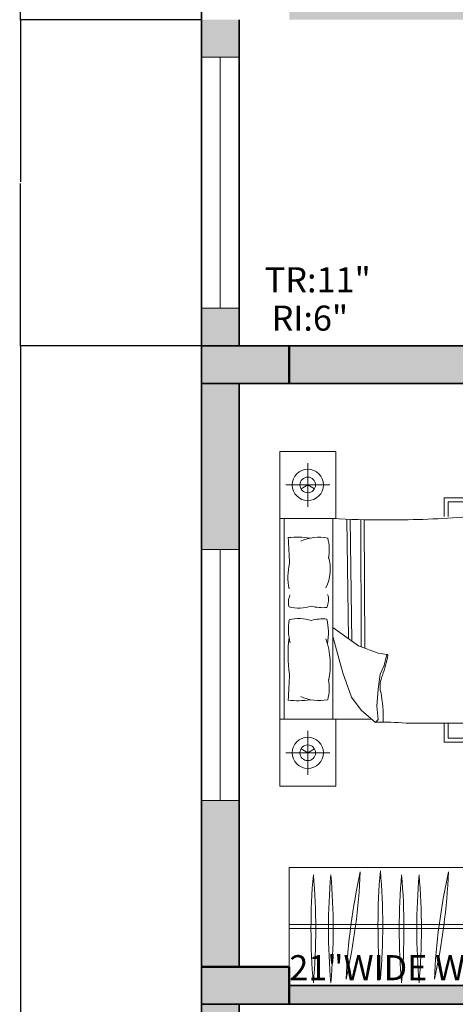
# Model space of a CAD drawing. Units: inches. Extents: x -28 to 485, y -861 to 54.
# Tile 2 of 14: x -28 to 76, y -600 to -365. Entities that reach past the tile are written whole.
import ezdxf

# ---------------------------------------------------------------- set-up
doc = ezdxf.new("R2010")
doc.units = ezdxf.units.IN
doc.header["$MEASUREMENT"] = 0
for name, color, linetype, lineweight in [('A-ANNO-DIMS', 2, 'Continuous', 18), ('A-ANNO-TEXT', 7, 'Continuous', 18), ('A-COLS', 7, 'Continuous', 50), ('A-COLS-PATT', 8, 'Continuous', 13), ('A-FLOR-CASE', 8, 'Continuous', 18), ('A-FURN', 8, 'Continuous', 13), ('A-GLAZ', 4, 'Continuous', 18), ('A-WALL', 7, 'Continuous', 35), ('A-WALL-PATT', 34, 'Continuous', 13)]:
    doc.layers.add(name, color=color, linetype=linetype, lineweight=lineweight)
doc.styles.get("Standard").update_dxf_attribs({"font": 'arial.ttf'})
doc.dimstyles.get("Standard").update_dxf_attribs({"dimtxt": 0.18, "dimasz": 0.18, "dimexe": 0.18, "dimexo": 0.0625, "dimgap": 0.09, "dimtad": 0, "dimtih": 1, "dimtoh": 1, "dimdec": 0, "dimzin": 0, "dimdsep": 46, "dimlunit": 3, "dimtxsty": 'Standard', "dimcen": 0.09, "dimadec": 0, "dimazin": 0, "dimtfac": 1, "dimtdec": 0, "dimtofl": 0, "dimtmove": 0, "dimatfit": 3, "dimfxl": 1, "dimtolj": 1, "dimtzin": 0, "dimarcsym": 0})

# ---------------------------------------------------------------- blocks, each defined once
blk = doc.blocks.new('BED-DOUBLE-WITH-NIGHTSTANDS')
for p, q in [((0, 0), (0, 80.08)), ((6.67, 66.84), (6.67, 77.31)), ((11.91, 72.08), (1.44, 72.08)), ((39.26, 64.51), (39.26, 68.96)), ((39.26, 68.96), (68.11, 68.96)), ((68.11, 68.96), (68.11, 10.57)), ((40.19, 68.03), (40.19, 64.5)), ((67.18, 68.03), (40.19, 68.03)), ((67.18, 11.5), (67.18, 68.03)), ((1.03, 64.07), (1.03, 16.02)), ((12.66, 16.02), (12.66, 64.07)), ((15.98, 63.85), (16.38, 35.34)), ((16.8, 63.82), (17.22, 34.74)), ((19.33, 63.78), (19.45, 33.37)), ((20.15, 63.78), (20.27, 33.06)), ((44.25, 64.43), (44.25, 15.09)), ((45.25, 64.51), (45.25, 15.09)), ((59.06, 60.14), (58.15, 60.31)), ((53.12, 56.3), (53.12, 23.78)), ((59.06, 54.54), (58.15, 54.36)), ((12.66, 38.02), (18.76, 33.63)), ((15.04, 27.14), (12.66, 35.87)), ((18.76, 33.63), (23.47, 31.84)), ((23.47, 31.84), (25.57, 31.52)), ((25.57, 31.52), (24.92, 28.93)), ((24.92, 28.93), (23.95, 26.82)), ((17.14, 21.3), (15.04, 27.14)), ((23.95, 26.82), (23.47, 23.25)), ((59.06, 24.99), (58.15, 25.16)), ((19.41, 18.22), (17.14, 21.3)), ((23.47, 23.25), (23.14, 19.19)), ((23.14, 19.19), (23.47, 15.95)), ((59.06, 19.39), (58.15, 19.21)), ((22.82, 15.3), (19.41, 18.22)), ((0, 16.02), (21.98, 16.02)), ((23.47, 15.95), (22.82, 15.3)), ((39.26, 10.57), (39.26, 15.1)), ((40.19, 15.1), (40.19, 11.5)), ((6.67, 13.24), (6.67, 2.78)), ((68.11, 10.57), (39.26, 10.57)), ((40.19, 11.5), (67.18, 11.5)), ((11.91, 8.01), (1.44, 8.01))]:
    blk.add_line(p, q)
for points in [[(0, 64.07), (13.35, 64.07), (13.35, 80.08), (0, 80.08)], [(6.67, 72.08), (5.06, 71.14)], [(6.67, 72.08), (8.29, 71.14)], [(13.35, 16.02), (13.35, 0), (0, 0)], [(6.67, 8.01), (5.06, 8.94)], [(6.67, 8.01), (8.29, 8.94)]]:
    blk.add_lwpolyline(points)
for points in [[(43.62, 64.41, 0.056112), (48.03, 64.99, 0.095341), (52.27, 66.12)], [(2, 59.47, -0.074897), (7.23, 59.37, 0.472817)], [(7.52, 43.09, -0.14099), (2.18, 42.93, -0.235245)], [(7.52, 39.67, 0.14099), (2.18, 39.83, 0.235245)], [(2, 20.62, 0.074897), (7.23, 20.71, -0.472817)], [(30.15, 15.13, 0.001242), (45.35, 15.09, -0.127202), (52.92, 13.49)]]:
    blk.add_lwpolyline(points, format="xyb")
for centre, radius in [((6.67, 72.08), 3.74), ((6.67, 72.08), 1.87), ((64.11, 56.84), 0.204), ((61.96, 55.51), 0.204), ((61.96, 24.02), 0.204), ((64.11, 22.68), 0.204), ((6.67, 8.01), 3.74), ((6.67, 8.01), 1.87)]:
    blk.add_circle(centre, radius)
for centre, radius, start, end in [((52.68, 65.51), 0.73, 336.5219, 123.8264), ((69.62, 57.92), 10.46, 111.4092, 145.6135), ((68.59, 75.81), 10.46, 228.1144, 262.255), ((69.99, 70.57), 5.1, 209.8884, 236.5383), ((70.94, 72.4), 6.35, 223.5186, 233.6964), ((22.44, 207.63), 143.9, 266.1, 270.9282), ((27.68, 251.44), 187.71, 269.1145, 274.8735), ((131.01, 58.75), 77.93, 175.2402, 181.8035), ((60.79, 62.99), 0.867, 76.272, 177.0484), ((59.47, 64.76), 1.79, 284.7031, 328.6173), ((61.96, 62.49), 1.65, 125.7657, 194.5347), ((53.85, 65.41), 7.32, 332.8176, 347.4827), ((61.24, 62.69), 1.16, 20.9613, 102.2885), ((61.86, 63.85), 0.873, 181.7131, 301.5367), ((59, 62.09), 2.64, 2.0648, 41.1598), ((60.59, 63.07), 0.856, 316.2238, 62.3173), ((68.81, 67.71), 4.25, 221.0454, 247.4453), ((66.52, 79.36), 14.47, 266.3481, 272.5919), ((58.76, 65.61), 6.06, 203.6453, 236.3329), ((55.85, 62.08), 1.35, 88.9462, 185.5144), ((56.85, 62.5), 2.41, 193.079, 274.7067), ((56.04, 61.53), 1.91, 7.1143, 95.0551), ((55.32, 60.77), 1.86, 338.5779, 68.4181), ((55.62, 61.86), 2.33, 305.9599, 357.6409), ((56.48, 64.35), 3.78, 288.2955, 328.7386), ((59.12, 61.97), 1.2, 19.1312, 189.736), ((58.76, 62.26), 1.5, 285.6955, 4.031), ((60.76, 60.64), 1.6, 128.4175, 173.8338), ((60.43, 62.21), 0.737, 126.7319, 206.0245), ((61.09, 62.57), 0.0682, 20.2667, 316.2271), ((61.51, 62.18), 0.13, 168.5166, 2.0648), ((61.45, 62.19), 0.0631, 52.0591, 168.5166), ((-760.15, 15.33), 763.42, 2.85022, 3.31479), ((9.33, 49.26), 10.32, 78.2417, 114.8684), ((1.06, 56.61), 10.73, 348.9631, 14.8961), ((54, 59.28), 0.964, 127.675, 162.5814), ((54, 59.28), 0.964, 196.6343, 225.5483), ((53.71, 63.39), 3.32, 259.249, 301.1782), ((54.57, 60.82), 2.55, 240.8249, 340.7178), ((53.81, 59.69), 1.2, 246.1646, 318.4347), ((55.15, 57.49), 3.09, 85.2696, 124.215), ((55.03, 61.2), 2.3, 240.0851, 262.564), ((55.94, 57.8), 1.64, 74.8529, 138.4347), ((57.33, 61.13), 1.99, 196.8663, 330.0915), ((56.5, 59.87), 0.497, 254.8529, 12.6959), ((55.15, 57.49), 3.09, 53.6555, 57.2989), ((56.78, 64.39), 4.3, 273.4924, 303.7117), ((60.19, 59.12), 0.158, 125.0752, 284.7644), ((60.43, 59.18), 0.34, 127.3642, 168.4363), ((60.17, 59.45), 0.49, 277.4968, 341.2737), ((60.56, 59.22), 0.195, 88.1325, 178.8919), ((60.95, 59.02), 0.422, 136.3462, 189.6513), ((60.71, 58.98), 0.176, 189.6513, 312.3208), ((60.75, 59.46), 0.204, 183.2768, 356.7232), ((61.39, 59.1), 0.668, 164.2829, 186.9148), ((60.6, 59.09), 0.334, 312.3208, 40.2111), ((61.31, 59.47), 0.474, 201.6382, 274.947), ((60.68, 58.82), 0.619, 42.3896, 66.5724), ((66.93, 63.72), 7.6, 217.9541, 226.8459), ((61.13, 59.18), 0.337, 10.9597, 52.2379), ((61.33, 59.15), 0.156, 274.947, 37.5263), ((57.16, 57.12), 0.251, 169.5864, 349.5616), ((57.25, 57.11), 0.154, 349.5616, 167.2949), ((61.28, 51.56), 6.63, 110.1059, 116.9968), ((59.06, 57.02), 0.42, 129.5056, 182.6421), ((57.85, 58), 1.27, 308.4388, 328.836), ((57.63, 59.02), 2.26, 296.5064, 305.3102), ((57.61, 57.86), 1.29, 336.3901, 344.4871), ((59.01, 57.53), 0.163, 83.9457, 185.6216), ((58.36, 57.69), 0.671, 328.836, 0.8141), ((58.71, 57.49), 0.384, 306.5232, 32.4668), ((59.16, 57.79), 0.163, 112.5583, 214.2343), ((59.06, 58.08), 0.384, 265.7131, 351.6568), ((58.72, 58.29), 0.671, 297.3659, 329.344), ((58.21, 58.87), 1.29, 313.6929, 321.7899), ((59.64, 57.99), 0.42, 115.5379, 168.6744), ((58.21, 58.6), 1.27, 329.344, 349.7412), ((61.28, 51.56), 6.63, 86.1723, 106.4158), ((57.2, 58.31), 2.26, 352.8698, 1.6736), ((61.66, 57.07), 0.93, 253.6301, 325.4631), ((61.86, 58.27), 0.163, 112.5583, 214.2343), ((61.75, 58.56), 0.384, 265.7131, 351.6568), ((61.42, 58.77), 0.671, 297.3659, 329.344), ((61.45, 54.86), 3.33, 60.7959, 85.244), ((54.37, 50.07), 10.94, 37.8256, 47.7588), ((60.91, 59.35), 1.29, 313.6929, 321.7899), ((61.87, 56.57), 0.565, 273.8774, 357.1501), ((62.33, 58.47), 0.42, 115.5379, 168.6744), ((60.9, 59.07), 1.27, 329.344, 349.7412), ((62.09, 56.97), 0.547, 262.0748, 308.2393), ((59.89, 58.78), 2.26, 352.8698, 1.6736), ((62.87, 56.86), 0.547, 215.1128, 261.2773), ((63.31, 56.83), 0.93, 197.889, 269.722), ((65.87, 54.52), 3.99, 130.182, 149.456), ((63.07, 58.33), 0.228, 33.0979, 123.1364), ((58.05, 55.12), 5.96, 31.1156, 34.8118), ((62.74, 57.94), 0.617, 2.3172, 70.5201), ((63.67, 56.79), 0.658, 139.3812, 199.9959), ((62.44, 57.27), 0.93, 310.9365, 22.7695), ((62.87, 57.22), 0.675, 285.6484, 332.2957), ((63.25, 57.78), 0.178, 135.7354, 318.1297), ((62.95, 58.07), 0.236, 315.7354, 31.1156), ((62.75, 57.57), 0.547, 319.3812, 5.5456), ((63.38, 57.79), 0.178, 68.2452, 250.6395), ((62.97, 58), 0.531, 352.6008, 57.1845), ((64.87, 54.44), 3.55, 111.7087, 116.2181), ((61.45, 54.86), 3.33, 47.5083, 55.9967), ((63.48, 58.12), 0.531, 252.8042, 349.6943), ((62.97, 57.17), 0.565, 331.1838, 51.6792), ((63.55, 56.5), 0.158, 125.0752, 284.7644), ((63.53, 58.17), 0.236, 248.2452, 323.6254), ((63.8, 56.56), 0.34, 93.635, 168.4363), ((63.33, 58.31), 0.617, 291.7087, 3.0299), ((63.75, 57.1), 0.2, 138.2946, 276.2474), ((63.53, 56.83), 0.49, 277.4968, 341.2737), ((63.83, 57.07), 0.278, 358.5719, 143.8954), ((58.93, 61.56), 5.96, 323.6254, 327.3216), ((63.92, 56.61), 0.195, 88.1325, 178.8919), ((63.99, 57.29), 0.281, 208.8493, 269.9355), ((63.75, 57.22), 0.321, 274.2123, 318.1587), ((64.31, 56.4), 0.422, 136.3462, 189.6513), ((63.81, 58.16), 0.228, 325.6077, 55.6462), ((64.75, 56.48), 0.668, 164.2829, 186.9148), ((64.73, 56.9), 0.643, 121.9501, 165.2442), ((63.96, 56.47), 0.334, 312.3208, 40.2111), ((64.67, 56.85), 0.474, 201.6382, 274.947), ((64.28, 57.14), 0.135, 262.868, 7.094), ((64.04, 56.2), 0.619, 42.3896, 66.5724), ((64.27, 57.26), 0.403, 278.5614, 22.5914), ((64.49, 56.56), 0.337, 10.9597, 118.7804), ((64.49, 57.27), 0.202, 44.3732, 121.9501), ((64.7, 56.53), 0.156, 274.947, 37.5263), ((1.85, 51.98), 10.19, 333.8761, 16.1746), ((54, 55.39), 0.964, 134.4517, 156.7144), ((54, 55.39), 0.964, 203.2856, 232.325), ((53.71, 51.28), 3.32, 58.8218, 100.2867), ((54.57, 53.85), 2.55, 19.2822, 119.1751), ((53.81, 54.99), 1.2, 41.5653, 113.8354), ((55.15, 57.18), 3.09, 235.785, 274.7304), ((55.03, 53.47), 2.3, 97.436, 119.9149), ((56.85, 52.18), 2.41, 85.2933, 166.921), ((55.94, 56.87), 1.64, 221.5653, 285.1471), ((57.33, 53.55), 1.99, 29.9085, 163.1337), ((55.32, 53.9), 1.86, 291.5819, 21.4221), ((56.5, 54.81), 0.497, 347.3041, 105.1471), ((55.15, 57.18), 3.09, 302.7011, 306.3445), ((55.62, 52.81), 2.33, 2.3591, 54.0401), ((56.78, 50.29), 4.3, 56.2883, 86.5076), ((61.4, 55.17), 0.158, 125.0752, 284.7644), ((61.65, 55.23), 0.34, 93.635, 168.4363), ((61.92, 55.78), 0.658, 82.0748, 142.6895), ((61.85, 56.68), 0.675, 228.342, 274.9894), ((61.6, 55.76), 0.2, 138.2946, 276.2474), ((61.38, 55.5), 0.49, 277.4968, 341.2737), ((61.68, 55.73), 0.278, 358.5719, 143.8954), ((61.77, 55.27), 0.195, 88.1325, 178.8919), ((61.84, 55.95), 0.281, 208.8493, 269.9355), ((61.6, 55.89), 0.321, 274.2123, 318.1587), ((62.16, 55.06), 0.422, 136.3462, 189.6513), ((61.92, 55.02), 0.176, 189.6513, 312.3208), ((65.87, 54.52), 3.99, 175.2415, 182.8929), ((62.6, 55.14), 0.668, 164.2829, 186.9148), ((62.58, 55.56), 0.643, 121.9501, 165.2442), ((61.81, 55.14), 0.334, 312.3208, 40.2111), ((62.52, 55.52), 0.474, 201.6382, 274.947), ((62.13, 55.81), 0.135, 262.868, 7.094), ((61.89, 54.87), 0.619, 42.3896, 66.5724), ((62.12, 55.92), 0.403, 278.5614, 22.5914), ((62.34, 55.23), 0.337, 10.9597, 118.7804), ((65.87, 54.52), 3.99, 156.1523, 156.9499), ((62.34, 55.94), 0.202, 44.3732, 121.9501), ((62.97, 56.41), 0.565, 181.4625, 249.4747), ((62.55, 55.2), 0.156, 274.947, 37.5263), ((63.02, 56.51), 0.675, 248.3627, 295.0101), ((62.69, 55.67), 0.658, 20.6625, 81.2773), ((64.07, 56.36), 0.176, 189.6513, 312.3208), ((16.01, 49.96), 14.08, 166.3427, 191.1841), ((58.76, 49.06), 6.06, 123.6671, 158.5059), ((55.85, 52.59), 1.35, 174.4856, 271.0538), ((56.04, 53.15), 1.91, 264.9449, 352.8857), ((56.48, 50.32), 3.78, 31.2614, 71.7045), ((59.12, 52.71), 1.2, 170.264, 340.8688), ((60.76, 54.03), 1.6, 186.1662, 231.5825), ((58.76, 52.42), 1.5, 355.969, 74.3045), ((60.43, 52.46), 0.737, 153.9755, 233.2681), ((61.96, 52.19), 1.65, 165.4653, 234.2343), ((53.85, 49.26), 7.32, 12.5173, 27.1824), ((59, 52.59), 2.64, 318.8402, 357.9352), ((60.59, 51.6), 0.856, 297.6827, 43.7762), ((61.13, 52.12), 0.113, 43.7762, 339.7183), ((61.51, 52.5), 0.13, 357.9352, 191.4834), ((61.45, 52.48), 0.0631, 191.4834, 307.9409), ((60.79, 51.69), 0.867, 182.9516, 283.728), ((59.47, 49.92), 1.79, 31.3827, 75.2969), ((61.86, 50.82), 0.873, 58.4633, 178.2869), ((61.24, 51.98), 1.16, 257.7115, 339.0387), ((69.62, 56.75), 10.46, 214.3865, 248.5908), ((68.81, 46.96), 4.25, 112.5547, 138.9546), ((66.52, 35.31), 14.47, 87.4081, 93.6519), ((66.17, 41.19), 8.09, 82.8636, 171.8197), ((74.19, 42.33), 10.46, 152.5854, 175.5377), ((66.74, 46.53), 1.88, 76.3898, 169.0739), ((66.48, 45.12), 2.37, 72.8609, 131.9049), ((5.99, 44.03), 3.96, 153.3437, 196.1026), ((7.37, 44.56), 4.25, 335.0183, 18.5407), ((65.43, 42.24), 4.68, 68.117, 96.6195), ((72.68, 45.26), 5.75, 162.9798, 196.4569), ((10.2, 52.53), 9.81, 254.1707, 275.9871), ((58.94, 41.49), 1.16, 50.8855, 132.2127), ((64.01, 42.31), 0.867, 106.1963, 206.9726), ((61.98, 43.19), 1.79, 314.6273, 358.5415), ((65.27, 42.46), 1.65, 155.6899, 224.4589), ((64.54, 42.29), 1.16, 50.8855, 132.2127), ((64.51, 43.6), 0.873, 211.6373, 331.4609), ((63.8, 42.29), 0.856, 346.148, 92.2415), ((62.91, 40.64), 2.64, 31.989, 71.0841), ((56.78, 40.96), 7.32, 2.7418, 17.407), ((75.64, 42.98), 8.5, 174.3643, 175.6213), ((81.47, 38.5), 15.2, 160.0972, 160.2783), ((10.2, 30.23), 9.81, 84.0129, 105.8293), ((58.4, 41.51), 0.867, 106.1963, 206.9726), ((58.4, 40.68), 0.867, 153.0274, 253.8037), ((56.38, 42.39), 1.79, 314.6273, 358.5415), ((56.38, 39.81), 1.79, 1.4585, 45.3727), ((59.67, 41.66), 1.65, 155.6899, 224.4589), ((59.67, 40.53), 1.65, 135.5411, 204.3101), ((58.91, 42.8), 0.873, 211.6373, 331.4609), ((58.2, 41.49), 0.856, 346.148, 92.2415), ((57.3, 39.84), 2.64, 31.989, 71.0841), ((51.18, 40.16), 7.32, 2.7418, 17.407), ((51.18, 42.04), 7.32, 342.593, 357.2582), ((57.3, 42.35), 2.64, 288.9159, 328.011), ((58.2, 40.71), 0.856, 267.7585, 13.852), ((58.91, 39.39), 0.873, 28.5391, 148.3627), ((58.87, 41.3), 0.0682, 50.1909, 346.0209), ((58.92, 40.88), 0.113, 13.852, 309.9245), ((59.44, 41.17), 0.13, 198.4408, 31.989), ((59.37, 41.15), 0.0631, 81.9833, 198.4408), ((59.44, 41.02), 0.13, 328.011, 161.5592), ((59.37, 41.04), 0.0631, 161.5592, 278.0167), ((64.01, 39.88), 0.867, 153.0274, 253.8037), ((61.98, 39.01), 1.79, 1.4585, 45.3727), ((65.27, 39.73), 1.65, 135.5411, 204.3101), ((56.78, 41.24), 7.32, 342.593, 357.2582), ((62.91, 41.55), 2.64, 288.9159, 328.011), ((63.8, 39.91), 0.856, 267.7585, 13.852), ((64.52, 40.08), 0.113, 13.852, 309.9245), ((64.47, 42.1), 0.0682, 50.1909, 346.0209), ((64.98, 41.95), 0.0631, 81.9833, 198.4408), ((64.98, 40.24), 0.0631, 161.5592, 278.0167), ((65.04, 41.98), 0.13, 198.4408, 31.989), ((65.04, 40.22), 0.13, 328.011, 161.5592), ((16.3, 37.72), 14.27, 171.5249, 193.96), ((-2.51, 36.66), 14.12, 349.8617, 13.6238), ((58.94, 40.71), 1.16, 227.7873, 309.1145), ((68.59, 40.66), 10.46, 184.4623, 262.255), ((64.51, 38.59), 0.873, 28.5391, 148.3627), ((64.54, 39.91), 1.16, 227.7873, 309.1145), ((74.19, 39.86), 10.46, 184.4623, 207.4146), ((72.68, 36.94), 5.75, 163.5431, 197.0202), ((75.64, 39.22), 8.5, 184.3787, 185.6357), ((81.47, 43.7), 15.2, 199.7217, 199.9028), ((30.98, 31.59), 29.04, 172.2196, 189.497), ((-6.57, 29.12), 18.61, 348.0397, 19.2615), ((69.99, 35.42), 5.1, 181.272, 236.5383), ((72.72, 40.59), 9.45, 214.0123, 234.053), ((70.94, 37.25), 6.35, 197.8504, 233.6964), ((-4.69, 37.08), 31.06, 340.1194, 349.3383), ((25.64, 31.34), 0.193, 358.8623, 109.7536), ((69.62, 22.77), 10.46, 111.4092, 145.6135), ((55.85, 26.93), 1.35, 88.9462, 185.5144), ((56.04, 26.38), 1.91, 7.1143, 95.0551), ((60.79, 27.84), 0.867, 76.272, 177.0484), ((59.47, 29.61), 1.79, 284.7031, 328.6173), ((61.96, 27.34), 1.65, 125.7657, 194.5347), ((53.85, 30.27), 7.32, 332.8176, 347.4827), ((61.24, 27.55), 1.16, 20.9613, 102.2885), ((60.59, 27.92), 0.856, 316.2238, 62.3173), ((59, 26.94), 2.64, 2.0648, 41.1598), ((61.86, 28.71), 0.873, 181.7131, 301.5367), ((66.52, 44.21), 14.47, 266.3481, 272.5919), ((68.81, 32.56), 4.25, 221.0454, 247.4453), ((-760.15, 64.76), 763.42, 356.68521, 357.14978), ((30.48, 23.89), 6.52, 156.2616, 191.3392), ((58.76, 30.46), 6.06, 201.4941, 236.3329), ((56.85, 27.35), 2.41, 193.079, 274.7067), ((55.32, 25.63), 1.86, 338.5779, 68.4181), ((55.62, 26.71), 2.33, 305.9599, 357.6409), ((56.48, 29.2), 3.78, 288.2955, 328.7386), ((59.12, 26.82), 1.2, 19.1312, 189.736), ((58.76, 27.11), 1.5, 285.6955, 4.031), ((60.76, 25.49), 1.6, 128.4175, 173.8338), ((60.43, 27.07), 0.737, 126.7319, 206.0245), ((61.09, 27.42), 0.0682, 20.2667, 316.2271), ((61.51, 27.03), 0.13, 168.5166, 2.0648), ((61.45, 27.04), 0.0631, 52.0591, 168.5166), ((1.06, 23.47), 10.73, 345.1039, 11.0369), ((136.48, 22.83), 83.37, 179.3433, 185.6887), ((53.71, 28.24), 3.32, 259.7133, 301.1782), ((54, 24.13), 0.964, 127.675, 156.7144), ((54, 24.13), 0.964, 203.229, 225.5483), ((54.57, 25.67), 2.55, 240.8249, 340.7178), ((53.81, 24.54), 1.2, 246.1646, 318.4347), ((55.15, 22.34), 3.09, 85.2696, 124.215), ((55.03, 26.06), 2.3, 240.0851, 262.564), ((55.94, 22.65), 1.64, 74.8529, 138.4347), ((57.33, 25.98), 1.99, 196.8663, 330.0915), ((56.5, 24.72), 0.497, 254.8529, 12.6959), ((55.15, 22.34), 3.09, 53.6555, 57.2989), ((56.78, 29.24), 4.3, 273.4924, 303.7117), ((61.4, 24.36), 0.158, 75.2356, 234.9248), ((61.65, 24.3), 0.34, 191.5637, 266.365), ((61.6, 23.76), 0.2, 83.7526, 221.7054), ((61.38, 24.03), 0.49, 18.7263, 82.5032), ((61.68, 23.79), 0.278, 216.1046, 1.4281), ((61.77, 24.25), 0.195, 181.1081, 271.8675), ((61.84, 23.57), 0.281, 90.0645, 151.1507), ((61.6, 23.64), 0.321, 41.8413, 85.7877), ((61.92, 24.5), 0.176, 47.6792, 170.3487), ((62.16, 24.46), 0.422, 170.3487, 223.6538), ((65.87, 25.01), 3.99, 177.1071, 184.7585), ((62.6, 24.38), 0.668, 173.0852, 195.7171), ((62.58, 23.96), 0.643, 194.7558, 238.0499), ((61.81, 24.39), 0.334, 319.7889, 47.6792), ((62.52, 24.01), 0.474, 85.053, 158.3618), ((62.13, 23.71), 0.135, 352.906, 97.132), ((61.89, 24.66), 0.619, 293.4276, 317.6104), ((62.34, 24.29), 0.337, 241.2196, 349.0403), ((62.12, 23.6), 0.403, 337.4086, 81.4386), ((62.97, 23.11), 0.565, 110.5253, 178.5375), ((63.31, 22.7), 0.93, 90.278, 162.111), ((62.55, 24.33), 0.156, 322.4737, 85.053), ((63.02, 23.01), 0.675, 64.9899, 111.6373), ((62.69, 23.86), 0.658, 278.7227, 339.3375), ((9.33, 30.82), 10.32, 245.1316, 281.7583), ((-5.54, 16.67), 30.23, 357.4519, 11.3392), ((54.57, 18.71), 2.55, 19.2822, 119.1751), ((57.16, 22.4), 0.251, 10.4384, 190.4136), ((57.25, 22.42), 0.154, 192.7051, 10.4384), ((61.28, 27.97), 6.63, 243.0032, 249.8941), ((57.85, 21.53), 1.27, 31.164, 51.5612), ((59.06, 22.5), 0.42, 177.3579, 230.4944), ((57.63, 20.5), 2.26, 54.6898, 63.4936), ((57.61, 21.66), 1.29, 15.5129, 23.6099), ((59.01, 21.99), 0.163, 174.3784, 276.0543), ((58.71, 22.03), 0.384, 327.5332, 53.4768), ((58.36, 21.84), 0.671, 359.1859, 31.164), ((59.16, 21.74), 0.163, 145.7657, 247.4417), ((59.06, 21.45), 0.384, 8.3432, 94.2869), ((58.72, 21.23), 0.671, 30.656, 62.6341), ((58.21, 20.66), 1.29, 38.2101, 46.3071), ((59.64, 21.53), 0.42, 191.3256, 244.4621), ((58.21, 20.93), 1.27, 10.2588, 30.656), ((61.28, 27.97), 6.63, 253.5842, 273.8277), ((57.2, 21.22), 2.26, 358.3264, 7.1302), ((66.93, 15.8), 7.6, 133.1541, 142.0459), ((61.85, 22.84), 0.675, 85.0106, 131.658), ((61.66, 22.46), 0.93, 34.5369, 106.3699), ((61.92, 23.75), 0.658, 217.3105, 277.9252), ((61.86, 21.26), 0.163, 145.7657, 247.4417), ((54.37, 29.45), 10.94, 312.2412, 322.1744), ((61.45, 24.67), 3.33, 274.756, 299.2041), ((61.75, 20.97), 0.384, 8.3432, 94.2869), ((61.42, 20.76), 0.671, 30.656, 62.6341), ((61.87, 22.95), 0.565, 2.8499, 86.1226), ((62.09, 22.55), 0.547, 51.7607, 97.9252), ((65.87, 25.01), 3.99, 203.0501, 203.8477), ((62.34, 23.59), 0.202, 238.0499, 315.6268), ((62.87, 22.67), 0.547, 98.7227, 144.8872), ((65.87, 25.01), 3.99, 210.544, 229.818), ((62.74, 21.59), 0.617, 289.4799, 357.6828), ((58.05, 24.41), 5.96, 325.1882, 328.8844), ((63.67, 22.74), 0.658, 160.0041, 220.6188), ((62.44, 22.26), 0.93, 337.2305, 49.0635), ((62.87, 22.31), 0.675, 27.7043, 74.3516), ((63.25, 21.74), 0.178, 41.8703, 224.2646), ((62.95, 21.45), 0.236, 328.8844, 44.2646), ((62.75, 21.95), 0.547, 354.4544, 40.6188), ((63.38, 21.74), 0.178, 109.3605, 291.7548), ((62.97, 21.52), 0.531, 302.8155, 7.3992), ((64.87, 25.09), 3.55, 243.7819, 248.2913), ((61.45, 24.67), 3.33, 304.0033, 312.4917), ((62.97, 22.35), 0.565, 308.3208, 28.8162), ((63.48, 21.4), 0.531, 10.3057, 107.1958), ((63.55, 23.03), 0.158, 75.2356, 234.9248), ((63.53, 21.36), 0.236, 36.3746, 111.7548), ((63.8, 22.96), 0.34, 191.5637, 266.365), ((63.75, 22.43), 0.2, 83.7526, 221.7054), ((63.33, 21.21), 0.617, 356.9701, 68.2913), ((63.53, 22.69), 0.49, 18.7263, 82.5032), ((63.83, 22.46), 0.278, 216.1046, 1.4281), ((63.92, 22.92), 0.195, 181.1081, 271.8675), ((58.93, 17.96), 5.96, 32.6784, 36.3746), ((63.99, 22.24), 0.281, 90.0645, 151.1507), ((63.75, 22.31), 0.321, 41.8413, 85.7877), ((64.07, 23.17), 0.176, 47.6792, 170.3487), ((64.31, 23.13), 0.422, 170.3487, 223.6538), ((63.81, 21.37), 0.228, 304.3538, 34.3923), ((64.75, 23.05), 0.668, 173.0852, 195.7171), ((64.73, 22.63), 0.643, 194.7558, 238.0499), ((63.96, 23.05), 0.334, 319.7889, 47.6792), ((64.67, 22.68), 0.474, 85.053, 158.3618), ((64.28, 22.38), 0.135, 352.906, 97.132), ((64.04, 23.32), 0.619, 293.4276, 317.6104), ((64.49, 22.96), 0.337, 241.2196, 349.0403), ((64.27, 22.27), 0.403, 337.4086, 81.4386), ((64.49, 22.25), 0.202, 238.0499, 315.6268), ((64.7, 22.99), 0.156, 322.4737, 85.053), ((54, 20.25), 0.964, 134.4517, 153.558), ((54, 20.25), 0.964, 210.0293, 232.325), ((53.71, 16.14), 3.32, 58.8218, 99.1554), ((53.81, 19.84), 1.2, 41.5653, 113.8354), ((58.76, 13.91), 6.06, 123.6671, 153.2997), ((55.15, 22.04), 3.09, 235.785, 274.7304), ((55.03, 18.32), 2.3, 97.436, 119.9149), ((56.85, 17.03), 2.41, 85.2933, 166.921), ((55.94, 21.72), 1.64, 221.5653, 285.1471), ((57.33, 18.4), 1.99, 29.9085, 163.1337), ((55.32, 18.75), 1.86, 291.5819, 21.4221), ((56.5, 19.66), 0.497, 347.3041, 105.1471), ((55.15, 22.04), 3.09, 302.7011, 306.3445), ((55.62, 17.67), 2.33, 2.3591, 54.0401), ((56.78, 15.14), 4.3, 56.2883, 86.5076), ((60.19, 20.41), 0.158, 75.2356, 234.9248), ((60.43, 20.35), 0.34, 191.5637, 232.6358), ((60.17, 20.07), 0.49, 18.7263, 82.5032), ((60.56, 20.3), 0.195, 181.1081, 271.8675), ((60.71, 20.55), 0.176, 47.6792, 170.3487), ((60.95, 20.51), 0.422, 170.3487, 223.6538), ((60.75, 20.06), 0.204, 3.2768, 176.7232), ((61.39, 20.43), 0.668, 173.0852, 195.7171), ((60.6, 20.43), 0.334, 319.7889, 47.6792), ((61.31, 20.06), 0.474, 85.053, 158.3618), ((60.68, 20.7), 0.619, 293.4276, 317.6104), ((61.13, 20.34), 0.337, 307.7621, 349.0403), ((61.33, 20.37), 0.156, 322.4737, 85.053), ((60.91, 20.18), 1.29, 38.2101, 46.3071), ((62.33, 21.06), 0.42, 191.3256, 244.4621), ((60.9, 20.45), 1.27, 10.2588, 30.656), ((59.89, 20.74), 2.26, 358.3264, 7.1302), ((63.07, 21.2), 0.228, 236.8636, 326.9021), ((55.85, 17.44), 1.35, 174.4856, 271.0538), ((56.04, 18), 1.91, 264.9449, 352.8857), ((56.48, 15.18), 3.78, 31.2614, 71.7045), ((59.12, 17.56), 1.2, 170.264, 340.8688), ((58.76, 17.27), 1.5, 355.969, 74.3045), ((60.76, 18.89), 1.6, 186.1662, 231.5825), ((60.43, 17.31), 0.737, 153.9755, 233.2681), ((59.47, 14.77), 1.79, 31.3827, 75.2969), ((60.79, 16.54), 0.867, 182.9516, 283.728), ((61.96, 17.04), 1.65, 165.4653, 234.2343), ((53.85, 14.11), 7.32, 12.5173, 27.1824), ((59, 17.44), 2.64, 318.8402, 357.9352), ((60.59, 16.46), 0.856, 297.6827, 43.7762), ((61.86, 15.67), 0.873, 58.4633, 178.2869), ((61.13, 16.97), 0.113, 43.7762, 339.7183), ((61.51, 17.35), 0.13, 357.9352, 191.4834), ((61.45, 17.33), 0.0631, 191.4834, 307.9409), ((24.81, -58.13), 73.46, 85.8294, 91.553), ((52.87, 14.23), 0.739, 273.98, 27.3412), ((61.24, 16.83), 1.16, 257.7115, 339.0387), ((69.62, 21.6), 10.46, 214.3865, 248.5908), ((68.81, 11.81), 4.25, 112.5547, 138.9546), ((66.52, 0.17), 14.47, 87.4081, 93.6519), ((68.59, 3.71), 10.46, 97.745, 131.8856), ((69.99, 8.96), 5.1, 123.4617, 150.1116), ((70.94, 7.13), 6.35, 126.3036, 136.4814)]:
    blk.add_arc(centre, radius, start, end)
blk = doc.blocks.new('WARDROBE-HANGING')
for p, q in [((84.7, 28.23), (0, 28.23)), ((0, 28.23), (0, 0)), ((84.7, 28.23), (84.7, 0)), ((84.7, 14.59), (0, 14.59)), ((84.7, 13.65), (0, 13.65)), ((84.7, 0), (0, 0))]:
    blk.add_line(p, q)
for centre, start, end in [((153.74, 13.55), 175.0028, 184.9972), ((-142.25, 13.55), 355.0028, 4.9972), ((157.93, 13.55), 175.0028, 184.9972), ((-138.07, 13.55), 355.0028, 4.9972), ((-131.46, 33.65), 347.508, 357.5023), ((162.01, -4.96), 167.508, 177.5023), ((169.76, 14.46), 175.0028, 184.9972), ((-126.23, 14.46), 355.0028, 4.9972), ((174.85, 13.55), 175.0028, 184.9972), ((-121.15, 13.55), 355.0028, 4.9972), ((179.03, 13.55), 175.0028, 184.9972), ((-116.97, 13.55), 355.0028, 4.9972), ((-110.36, 33.65), 347.508, 357.5023), ((183.11, -4.96), 167.508, 177.5023), ((190.86, 14.46), 175.0028, 184.9972), ((-105.13, 14.46), 355.0028, 4.9972), ((196.03, 13.55), 175.0028, 184.9972), ((-99.97, 13.55), 355.0028, 4.9972), ((200.21, 13.55), 175.0028, 184.9972), ((-95.78, 13.55), 355.0028, 4.9972), ((204.29, -4.96), 167.508, 177.5023), ((-89.17, 33.65), 347.508, 357.5023), ((212.05, 14.46), 175.0028, 184.9972), ((-83.95, 14.46), 355.0028, 4.9972), ((217.13, 13.55), 175.0028, 184.9972), ((-78.86, 13.55), 355.0028, 4.9972), ((221.31, 13.55), 175.0028, 184.9972), ((-74.68, 13.55), 355.0028, 4.9972), ((225.4, -4.96), 167.508, 177.5023), ((-68.07, 33.65), 347.508, 357.5023)]:
    blk.add_arc(centre, 148.56, start, end)
blk = doc.blocks.new('WINDOW-60IN')
for p, q in [((0, 60), (0, 0)), ((9, 60), (0, 60)), ((4.5, 60), (4.5, 0)), ((9, 0), (9, 60)), ((0, 0), (9, 0))]:
    blk.add_line(p, q)
blk = doc.blocks.new('*D54')
at = {"layer": 'A-ANNO-DIMS', "color": 0, "lineweight": -2, "transparency": 16777216}
for p, q in [((15.22, 10.13), (-28.15, 10.13)), ((-27.97, 9.95), (-27.97, -177.18)), ((-27.97, -364.69), (-27.97, -177.55)), ((15.22, -364.87), (-28.15, -364.87))]:
    blk.add_line(p, q, dxfattribs=at)
at = {"layer": 'A-ANNO-DIMS', "color": 0, "transparency": 16777216}
for points in [[(-28, 9.95), (-27.94, 9.95), (-27.97, 10.13)], [(-28, -364.69), (-27.94, -364.69), (-27.97, -364.87)]]:
    blk.add_solid(points, dxfattribs=at)
at = {"layer": 'Defpoints', "color": 0, "transparency": 16777216}
for p in [(15.28, 10.13), (-27.97, -364.87), (15.28, -364.87)]:
    blk.add_point(p, dxfattribs=at)
at = {"layer": 'A-ANNO-DIMS', "color": 0, "transparency": 16777216, "insert": (-27.97, -177.37), "char_height": 0.18, "attachment_point": 5}
blk.add_mtext('\\A1;375', dxfattribs=at)
blk = doc.blocks.new('*D55')
at = {"layer": 'A-ANNO-DIMS', "color": 0, "lineweight": -2, "transparency": 16777216}
for p, q in [((15.22, -364.87), (-28.15, -364.87)), ((-27.97, -365.05), (-27.97, -403.68)), ((-27.97, -442.69), (-27.97, -404.05)), ((15.22, -442.87), (-28.15, -442.87))]:
    blk.add_line(p, q, dxfattribs=at)
at = {"layer": 'A-ANNO-DIMS', "color": 0, "transparency": 16777216}
for points in [[(-28, -365.05), (-27.94, -365.05), (-27.97, -364.87)], [(-28, -442.69), (-27.94, -442.69), (-27.97, -442.87)]]:
    blk.add_solid(points, dxfattribs=at)
at = {"layer": 'Defpoints', "color": 0, "transparency": 16777216}
for p in [(15.28, -364.87), (-27.97, -442.87), (15.28, -442.87)]:
    blk.add_point(p, dxfattribs=at)
at = {"layer": 'A-ANNO-DIMS', "color": 0, "transparency": 16777216, "insert": (-27.97, -403.87), "char_height": 0.18, "attachment_point": 5}
blk.add_mtext('\\A1;78', dxfattribs=at)
blk = doc.blocks.new('*D56')
at = {"layer": 'A-ANNO-DIMS', "color": 0, "lineweight": -2, "transparency": 16777216}
for p, q in [((15.22, -442.87), (-28.15, -442.87)), ((-27.97, -443.05), (-27.97, -630.18)), ((-27.97, -817.69), (-27.97, -630.55)), ((15.22, -817.87), (-28.15, -817.87))]:
    blk.add_line(p, q, dxfattribs=at)
at = {"layer": 'A-ANNO-DIMS', "color": 0, "transparency": 16777216}
for points in [[(-28, -443.05), (-27.94, -443.05), (-27.97, -442.87)], [(-28, -817.69), (-27.94, -817.69), (-27.97, -817.87)]]:
    blk.add_solid(points, dxfattribs=at)
at = {"layer": 'Defpoints', "color": 0, "transparency": 16777216}
for p in [(15.28, -442.87), (-27.97, -817.87), (15.28, -817.87)]:
    blk.add_point(p, dxfattribs=at)
at = {"layer": 'A-ANNO-DIMS', "color": 0, "transparency": 16777216, "insert": (-27.97, -630.37), "char_height": 0.18, "attachment_point": 5}
blk.add_mtext('\\A1;375', dxfattribs=at)

msp = doc.modelspace()

# ---------------------------------------------------------------- hatches: boundary and pattern name
at = {"layer": 'A-COLS-PATT'}
h = msp.add_hatch(color=256, dxfattribs=at)
h.dxf.hatch_style = 1
h.paths.add_polyline_path([(441.285, -591.367), (420.285, -591.367), (420.285, -595.867), (420.285, -600.367), (441.285, -600.367)])
h.paths.add_polyline_path([(304.691, -588.367), (295.785, -588.367), (295.785, -600.367), (304.691, -600.367)])
h.paths.add_polyline_path([(160.785, -588.367), (151.785, -588.367), (151.785, -600.367), (160.785, -600.367)])
h.paths.add_polyline_path([(36.285, -591.367), (24.285, -591.367), (15.285, -591.367), (15.285, -600.367), (36.285, -600.367)])
h.paths.add_polyline_path([(36.285, -808.867), (15.285, -808.867), (15.285, -817.867), (36.285, -817.867)])
h.paths.add_polyline_path([(160.785, -808.867), (139.785, -808.867), (139.785, -817.867), (160.785, -817.867)])
h.paths.add_polyline_path([(316.785, -808.867), (295.785, -808.867), (295.785, -817.867), (316.785, -817.867)])
h.paths.add_polyline_path([(441.285, -808.867), (420.285, -808.867), (420.285, -817.867), (441.285, -817.867)])
h.paths.add_polyline_path([(36.285, -442.867), (15.285, -442.867), (15.285, -451.867), (36.285, -451.867)])
h.paths.add_polyline_path([(160.785, -442.867), (139.785, -442.867), (139.785, -451.867), (160.785, -451.867)])
h.paths.add_polyline_path([(316.785, -442.867), (295.785, -442.867), (295.785, -451.867), (316.785, -451.867)])
h.paths.add_polyline_path([(441.285, -442.867), (420.285, -442.867), (420.285, -451.867), (441.285, -451.867)])
at = {"layer": 'A-WALL-PATT'}
h = msp.add_hatch(color=256, dxfattribs=at)
h.dxf.hatch_style = 1
h.paths.add_polyline_path([(160.785, -808.867), (160.785, -817.867), (295.785, -817.867), (295.785, -808.867)])
h.paths.add_polyline_path([(316.785, -817.867), (323.776, -817.867), (323.776, -808.867), (316.785, -808.867)])
h.paths.add_polyline_path([(420.285, -817.867), (420.285, -808.867), (383.776, -808.867), (383.776, -817.867)])
h.paths.add_polyline_path([(432.285, -808.867), (441.285, -808.867), (441.285, -702.966), (432.285, -702.966), (432.285, -708.367), (397.785, -708.367), (397.785, -710.617), (397.785, -712.867), (432.285, -712.867)])
h.paths.add_polyline_path([(300.285, -712.867), (329.285, -712.867), (329.285, -710.617), (329.285, -708.367), (295.785, -708.367), (295.785, -808.867), (300.285, -808.867)])
h.paths.add_polyline_path([(160.785, -698.867), (158.535, -698.867), (156.285, -698.867), (156.285, -808.867), (160.785, -808.867)])
h.paths.add_polyline_path([(36.285, -808.867), (36.285, -817.867), (79.721, -817.867), (79.721, -808.867)])
h.paths.add_polyline_path([(15.285, -808.867), (24.285, -808.867), (24.285, -739.09), (15.285, -739.09)])
h.paths.add_polyline_path([(24.285, -640.781), (15.285, -640.781), (15.285, -679.09), (24.285, -679.09), (24.285, -664.867), (89.285, -664.867), (89.285, -662.617), (89.285, -660.367), (24.285, -660.367)])
h.paths.add_polyline_path([(15.285, -616.781), (24.285, -616.781), (24.285, -600.367), (15.285, -600.367)])
h.paths.add_polyline_path([(36.285, -595.867), (36.285, -600.367), (123.285, -600.367), (123.285, -660.367), (117.285, -660.367), (117.285, -664.867), (156.285, -664.867), (156.285, -670.867), (160.785, -670.867), (160.785, -660.367), (127.785, -660.367), (127.785, -600.367), (129.785, -600.367), (129.785, -598.117), (129.785, -595.867)])
h.paths.add_polyline_path([(367.785, -664.867), (363.285, -664.867), (363.285, -708.367), (357.285, -708.367), (357.285, -712.867), (369.785, -712.867), (369.785, -708.367), (367.785, -708.367)])
h.paths.add_polyline_path([(432.285, -664.867), (432.285, -666.966), (441.285, -666.966), (441.285, -642.367), (432.285, -642.367), (432.285, -660.367), (328.785, -660.367), (328.785, -664.867), (363.285, -664.867)])
h.paths.add_polyline_path([(333.285, -600.367), (420.285, -600.367), (420.285, -595.867), (326.785, -595.867), (326.785, -600.367), (328.785, -600.367), (328.785, -630.367), (331.035, -630.367), (333.285, -630.367)])
h.paths.add_polyline_path([(441.285, -600.367), (432.285, -600.367), (432.285, -618.367), (441.285, -618.367)])
h.paths.add_polyline_path([(432.285, -591.367), (441.285, -591.367), (441.285, -547.793), (432.285, -547.793)])
h.paths.add_polyline_path([(295.785, -588.367), (300.238, -588.367), (300.285, -583.867), (300.285, -451.867), (295.785, -451.867)])
h.paths.add_polyline_path([(420.285, -451.867), (420.285, -442.867), (316.785, -442.867), (316.785, -451.867)])
h.paths.add_polyline_path([(432.285, -487.793), (441.285, -487.793), (441.285, -451.867), (432.285, -451.867)])
h.paths.add_polyline_path([(432.285, -442.867), (441.285, -442.867), (441.285, -364.867), (432.285, -364.867)])
h.paths.add_polyline_path([(261.785, -451.867), (261.785, -447.367), (261.785, -444.758), (261.785, -442.867), (160.785, -442.867), (160.785, -451.867)])
h.paths.add_polyline_path([(139.785, -451.867), (139.785, -442.867), (36.285, -442.867), (36.285, -451.867)])
h.paths.add_polyline_path([(15.285, -491.617), (24.285, -491.617), (24.285, -451.867), (15.285, -451.867)])
h.paths.add_polyline_path([(24.285, -551.617), (15.285, -551.617), (15.285, -591.367), (24.285, -591.367)])
h.paths.add_polyline_path([(160.785, -451.867), (156.285, -451.867), (156.285, -588.367), (160.785, -588.367)])
h.paths.add_polyline_path([(139.785, -364.867), (139.785, -355.867), (36.285, -355.867), (36.285, -364.867)])
h.paths.add_polyline_path([(24.285, -364.867), (15.285, -364.867), (15.285, -373.867), (24.285, -373.867)])
h.paths.add_polyline_path([(15.285, -433.867), (15.285, -442.867), (24.285, -442.867), (24.285, -433.867)])
h.paths.add_polyline_path([(261.785, -364.867), (261.785, -360.367), (261.785, -355.867), (160.785, -355.867), (160.785, -364.867)])
h.paths.add_polyline_path([(295.785, -355.867), (289.785, -355.867), (289.785, -364.867), (295.785, -364.867)])
h.paths.add_polyline_path([(295.785, -355.867), (300.285, -355.867), (300.285, -259.867), (333.285, -259.867), (333.285, -257.617), (333.285, -255.367), (300.285, -255.367), (300.285, -207.367), (295.785, -207.367)])
h.paths.add_polyline_path([(420.285, -364.867), (420.285, -355.867), (316.785, -355.867), (316.785, -364.867)])
h.paths.add_polyline_path([(24.285, -311.192), (15.285, -311.192), (15.285, -355.867), (24.285, -355.867)])
h.paths.add_polyline_path([(24.285, -211.867), (54.144, -211.867), (54.144, -207.367), (24.285, -207.367), (24.285, -187.772), (15.285, -187.772), (15.285, -251.192), (24.285, -251.192)])
h.paths.add_polyline_path([(82.144, -207.367), (82.144, -209.617), (82.144, -211.867), (127.785, -211.867), (127.785, -147.367), (129.785, -147.367), (129.785, -145.117), (129.785, -142.867), (36.285, -142.867), (36.285, -147.367), (123.285, -147.367), (123.285, -207.367)])
h.paths.add_polyline_path([(160.785, -207.367), (156.285, -207.367), (156.285, -355.867), (160.785, -355.867)])
h.paths.add_polyline_path([(24.285, 1.133), (15.285, 1.133), (15.285, -54.408), (24.285, -54.408)])
h.paths.add_polyline_path([(36.285, 10.133), (36.285, 1.133), (70.235, 1.133), (70.235, 10.133)])
h.paths.add_polyline_path([(15.285, -138.367), (24.285, -138.367), (24.285, -114.408), (15.285, -114.408)])
h.paths.add_polyline_path([(24.285, -147.367), (15.285, -147.367), (15.285, -163.772), (24.285, -163.772)])
h.paths.add_polyline_path([(156.285, -130.867), (160.785, -130.867), (160.785, 1.133), (156.285, 1.133)])
h.paths.add_polyline_path([(130.235, 1.133), (139.785, 1.133), (139.785, 10.133), (130.235, 10.133)])
h.paths.add_polyline_path([(316.785, 10.133), (316.785, 1.133), (328.097, 1.133), (328.097, 10.133)])
h.paths.add_polyline_path([(300.285, 1.133), (295.785, 1.133), (295.785, -130.867), (300.285, -130.867)])
h.paths.add_polyline_path([(420.285, -147.367), (420.285, -142.867), (326.785, -142.867), (326.785, -145.117), (326.785, -147.367), (328.785, -147.367), (328.785, -177.367), (331.035, -177.367), (333.285, -177.367), (333.285, -147.367)])
h.paths.add_polyline_path([(333.285, -207.367), (333.285, -205.367), (328.785, -205.367), (328.785, -211.867), (363.285, -211.867), (363.285, -255.367), (361.285, -255.367), (361.285, -259.867), (369.785, -259.867), (369.785, -255.367), (367.785, -255.367), (367.785, -211.867), (432.285, -211.867), (432.285, -214.893), (441.285, -214.893), (441.285, -188.008), (432.285, -188.008), (432.285, -207.367)])
h.paths.add_polyline_path([(441.285, -250.893), (432.285, -250.893), (432.285, -255.367), (397.785, -255.367), (397.785, -257.617), (397.785, -259.867), (432.285, -259.867), (432.285, -355.867), (441.285, -355.867)])
h.paths.add_polyline_path([(432.285, -138.367), (441.285, -138.367), (441.285, -115.099), (432.285, -115.099)])
h.paths.add_polyline_path([(441.285, -147.367), (432.285, -147.367), (432.285, -164.008), (441.285, -164.008)])
h.paths.add_polyline_path([(420.285, 1.133), (420.285, 10.133), (388.097, 10.133), (388.097, 1.133)])
h.paths.add_polyline_path([(432.285, -55.099), (441.285, -55.099), (441.285, 1.133), (432.285, 1.133)])

# ---------------------------------------------------------------- linework, layer by layer
at = {"layer": 'A-COLS'}
for p, q in [((36.285, -442.867), (36.285, -451.867)), ((15.285, -591.367), (24.285, -591.367)), ((24.285, -591.367), (36.285, -591.367)), ((36.285, -591.367), (36.285, -600.367))]:
    msp.add_line(p, q, dxfattribs=at)
at = {"layer": 'A-WALL'}
for p, q in [((15.285, 10.133), (15.285, -817.867)), ((24.285, -364.867), (24.285, -442.867)), ((15.285, -442.867), (345.285, -442.867)), ((15.285, -451.867), (261.785, -451.867)), ((24.285, -451.867), (24.285, -591.367)), ((36.285, -595.867), (129.785, -595.867)), ((15.285, -600.367), (123.285, -600.367)), ((24.285, -600.367), (24.285, -660.367))]:
    msp.add_line(p, q, dxfattribs=at)

# ---------------------------------------------------------------- block references
at = {"layer": 'A-FLOR-CASE'}
msp.add_blockref('WARDROBE-HANGING', (36.285, -595.867), dxfattribs=at)
at = {"layer": 'A-FURN'}
msp.add_blockref('BED-DOUBLE-WITH-NIGHTSTANDS', (34.03, -548.225), dxfattribs=at)
at = {"layer": 'A-GLAZ'}
for p in [(15.285, -433.867), (15.285, -551.617)]:
    msp.add_blockref('WINDOW-60IN', p, dxfattribs=at)

# ---------------------------------------------------------------- texts
at = {"layer": 'A-ANNO-TEXT', "char_height": 6, "attachment_point": 1}
for s, insert in [('TR:11"', (30.416, -424.081)), ('RI:6"', (32.055, -433.248)), ('21"WIDE WARDROBE', (36.285, -588.609))]:
    msp.add_mtext(s, dxfattribs=dict(at, insert=insert))

# ---------------------------------------------------------------- dimensions: what is measured, and where the dimension line sits
at = {"layer": 'A-ANNO-DIMS'}
for base, p1, p2, picture, middle in [((-27.965, -364.867), (15.285, 10.133), (15.285, -364.867), '*D54', (-27.965, -177.367)), ((-27.965, -442.867), (15.285, -364.867), (15.285, -442.867), '*D55', (-27.965, -403.867)), ((-27.965, -817.867), (15.285, -442.867), (15.285, -817.867), '*D56', (-27.965, -630.367))]:
    dim = msp.add_linear_dim(base=base, p1=p1, p2=p2, angle=90, dimstyle='Standard', override={"dimdec": 0, "dimlfac": 1, "dimrnd": 0, "dimzin": 0, "dimdsep": 46, "dimlunit": 2}, dxfattribs=at)
    dim.commit()
    dim.dimension.update_dxf_attribs({"geometry": picture, "text_midpoint": middle})

doc.saveas('drawing.dxf')
